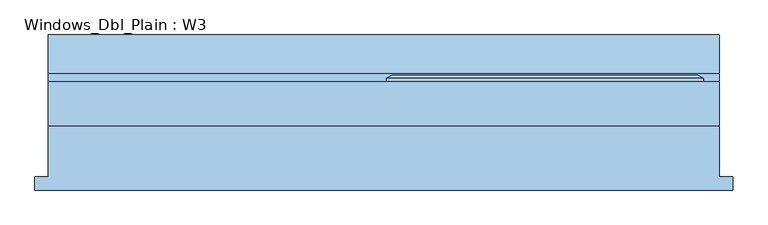
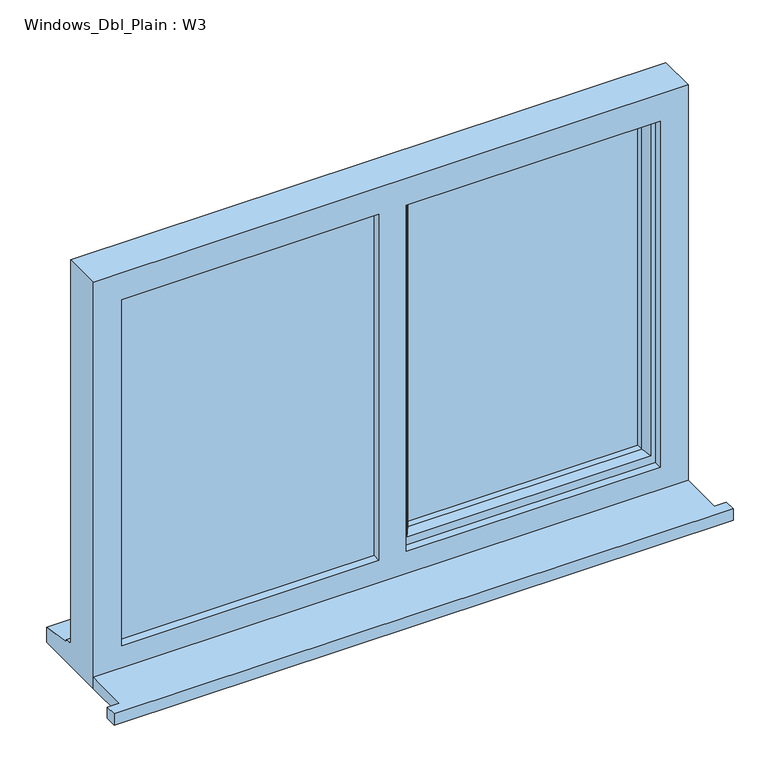
"""IFC4 building model written with IfcOpenShell, lengths in millimetres: window geometry, Windows_Dbl_Plain : W3."""

from ifc_helpers import new_model, si_unit, frame, origin, place, context, project, spatial, polyline, outline, extrude, faceted_brep, source, transform, mapped, element, save


def windows_dbl_plain_w3_a138f75b(model_context):
    return source(origin(), model_context, "Body", "SolidModel", [
        extrude(outline(polyline([(-940.3264, -130.8434322), (-940.3264, -105.8434322), (-915.3264, -105.8434322), (-915.3264, -10.2434322), (345.3264, -10.2434322), (345.3264, -105.8434322), (370.3264, -105.8434322), (370.3264, -130.8434322), (-940.3264, -130.8434322)])), frame((0.0, 0.0, 1200.0), z_axis=(0.0, 0.0, 1.0), x_axis=(1.0, 0.0, 0.0)), (0.0, 0.0, 1.0), 25.0),
        faceted_brep([(-280.0, 72.7565678, 2080.0), (-280.0, 78.5300705, 2080.0), (-280.0, 78.5300705, 1253.0), (-280.0, 72.7565678, 1253.0), (-270.0, 7.7565678, 2070.0), (-270.0, 72.7565678, 2070.0), (-270.0, 72.7565678, 1263.0), (-270.0, 7.7565678, 1263.0), (-230.0, 22.2494677, 2030.0), (-240.1480377, 7.7565678, 2040.1480377), (-240.1480377, 7.7565678, 1292.8519623), (-230.0, 22.2494677, 1303.0), (-230.0, 36.7565678, 2030.0), (-230.0, 36.7565678, 1303.0), (-240.0, 60.7565678, 2040.0), (-240.0, 36.7565678, 2040.0), (-240.0, 36.7565678, 1293.0), (-240.0, 60.7565678, 1293.0), (-230.0, 78.5300705, 2030.0), (-230.0, 60.7565678, 2030.0), (-230.0, 60.7565678, 1303.0), (-230.0, 78.5300705, 1303.0), (-247.4457548, 84.3035732, 2047.4457548), (-247.4457548, 84.3035732, 1285.5542452), (-269.2153903, 84.3035732, 2069.2153903), (-269.2153903, 84.3035732, 1263.7846097), (315.3264, 78.5300705, 1253.0), (315.3264, 72.7565678, 1253.0), (305.3264, 72.7565678, 1263.0), (305.3264, 7.7565678, 1263.0), (275.4744377, 7.7565678, 1292.8519623), (265.3264, 22.2494677, 1303.0), (265.3264, 36.7565678, 1303.0), (275.3264, 36.7565678, 1293.0), (275.3264, 60.7565678, 1293.0), (265.3264, 60.7565678, 1303.0), (265.3264, 78.5300705, 1303.0), (282.7721548, 84.3035732, 1285.5542452), (304.5417903, 84.3035732, 1263.7846097), (315.3264, 78.5300705, 2080.0), (315.3264, 72.7565678, 2080.0), (305.3264, 72.7565678, 2070.0), (305.3264, 7.7565678, 2070.0), (275.4744377, 7.7565678, 2040.1480377), (265.3264, 22.2494677, 2030.0), (265.3264, 36.7565678, 2030.0), (275.3264, 36.7565678, 2040.0), (275.3264, 60.7565678, 2040.0), (265.3264, 60.7565678, 2030.0), (265.3264, 78.5300705, 2030.0), (282.7721548, 84.3035732, 2047.4457548), (304.5417903, 84.3035732, 2069.2153903)], [[[0, 1, 2, 3]], [[4, 5, 6, 7]], [[8, 9, 10, 11]], [[12, 8, 11, 13]], [[14, 15, 16, 17]], [[18, 19, 20, 21]], [[22, 18, 21, 23]], [[1, 24, 25, 2]], [[3, 2, 26, 27]], [[7, 6, 28, 29]], [[11, 10, 30, 31]], [[13, 11, 31, 32]], [[17, 16, 33, 34]], [[21, 20, 35, 36]], [[23, 21, 36, 37]], [[2, 25, 38, 26]], [[27, 26, 39, 40]], [[29, 28, 41, 42]], [[31, 30, 43, 44]], [[32, 31, 44, 45]], [[34, 33, 46, 47]], [[36, 35, 48, 49]], [[37, 36, 49, 50]], [[26, 38, 51, 39]], [[40, 39, 1, 0]], [[3, 27, 40, 0], [5, 41, 28, 6]], [[42, 41, 5, 4]], [[7, 29, 42, 4], [9, 43, 30, 10]], [[44, 43, 9, 8]], [[45, 44, 8, 12]], [[15, 46, 33, 16], [13, 32, 45, 12]], [[47, 46, 15, 14]], [[17, 34, 47, 14], [19, 48, 35, 20]], [[49, 48, 19, 18]], [[50, 49, 18, 22]], [[24, 51, 38, 25], [23, 37, 50, 22]], [[39, 51, 24, 1]]]),
        extrude(outline(polyline([(2050.0, -310.0), (2070.0, -310.0), (2070.0, -875.3264), (1263.0, -875.3264), (1263.0, -310.0), (1283.0, -310.0), (1283.0, -855.3264), (2050.0, -855.3264), (2050.0, -310.0)])), frame((0.0, 31.7565678, 0.0), z_axis=(0.0, 1.0, 0.0), x_axis=(0.0, 0.0, 1.0)), (0.0, 0.0, 1.0), 41.0),
        faceted_brep([(345.3264, -10.2434322, 2110.0), (-915.3264, -10.2434322, 2110.0), (-915.3264, -10.2434322, 1200.0), (345.3264, -10.2434322, 1200.0), (285.3264, -10.2434322, 2050.0), (285.3264, -10.2434322, 1275.0), (-252.0, -10.2434322, 1275.0), (-252.0, -10.2434322, 2050.0), (-310.0, -10.2434322, 2050.0), (-310.0, -10.2434322, 1275.0), (-855.3264, -10.2434322, 1275.0), (-855.3264, -10.2434322, 2050.0), (-915.3264, 72.7565678, 2110.0), (-915.3264, 72.7565678, 1251.0), (-915.3264, 87.7565678, 1249.68767), (-915.3264, 87.7565678, 1244.7449676), (-915.3264, 160.2565678, 1233.8088847), (-915.3264, 160.2565678, 1200.0), (345.3264, 72.7565678, 2110.0), (345.3264, 72.7565678, 1251.0), (-875.3264, 72.7565678, 2070.0), (-875.3264, 72.7565678, 1263.0), (-310.0, 72.7565678, 1263.0), (-310.0, 72.7565678, 2070.0), (-270.0, 72.7565678, 2070.0), (-270.0, 72.7565678, 1263.0), (305.3264, 72.7565678, 1263.0), (305.3264, 72.7565678, 2070.0), (-875.3264, 7.7565678, 2070.0), (-875.3264, 7.7565678, 1263.0), (-300.0, 7.7565678, 2070.0), (-300.0, 7.7565678, 1263.0), (-310.0, 7.7565678, 2050.0), (-855.3264, 7.7565678, 2050.0), (-855.3264, 7.7565678, 1275.0), (-310.0, 7.7565678, 1275.0), (-270.0, 7.7565678, 2070.0), (305.3264, 7.7565678, 2070.0), (305.3264, 7.7565678, 1263.0), (-270.0, 7.7565678, 1263.0), (285.3264, 7.7565678, 2050.0), (-252.0, 7.7565678, 2050.0), (-252.0, 7.7565678, 1275.0), (285.3264, 7.7565678, 1275.0), (-310.0, 31.7565678, 2070.0), (-300.0, 31.7565678, 2070.0), (345.3264, 160.2565678, 1200.0), (345.3264, 160.2565678, 1233.8088847), (345.3264, 87.7565678, 1244.7449676), (345.3264, 87.7565678, 1249.68767), (-300.0, 31.7565678, 1263.0), (-310.0, 31.7565678, 1263.0)], [[[0, 1, 2, 3], [4, 5, 6, 7], [8, 9, 10, 11]], [[2, 1, 12, 13, 14, 15, 16, 17]], [[13, 12, 18, 19], [20, 21, 22, 23], [24, 25, 26, 27]], [[21, 20, 28, 29]], [[28, 30, 31, 29], [32, 33, 34, 35]], [[36, 37, 38, 39], [40, 41, 42, 43]], [[33, 11, 10, 34]], [[1, 0, 18, 12]], [[28, 20, 23, 44, 45, 30]], [[27, 37, 36, 24]], [[11, 33, 32, 8]], [[40, 4, 7, 41]], [[19, 18, 0, 3, 46, 47, 48, 49]], [[27, 26, 38, 37]], [[4, 40, 43, 5]], [[45, 50, 31, 30]], [[50, 45, 44, 51]], [[51, 44, 23, 22]], [[25, 24, 36, 39]], [[41, 7, 6, 42]], [[8, 32, 35, 9]], [[46, 3, 2, 17]], [[47, 46, 17, 16]], [[48, 47, 16, 15]], [[49, 48, 15, 14]], [[19, 49, 14, 13]], [[22, 21, 29, 31, 50, 51]], [[26, 25, 39, 38]], [[6, 5, 43, 42]], [[35, 34, 10, 9]]]),
        extrude(outline(polyline([(-875.3264, 31.7565678), (-300.0, 31.7565678), (-300.0, 7.7565678), (-875.3264, 7.7565678), (-875.3264, 31.7565678)])), frame((0.0, 0.0, 1263.0), z_axis=(0.0, 0.0, 1.0), x_axis=(1.0, 0.0, 0.0)), (0.0, 0.0, 1.0), 807.0),
        extrude(outline(polyline([(275.3264, 36.7565678), (-240.0, 36.7565678), (-240.0, 60.7565678), (275.3264, 60.7565678), (275.3264, 36.7565678)])), frame((0.0, 0.0, 1293.0), z_axis=(0.0, 0.0, 1.0), x_axis=(1.0, 0.0, 0.0)), (0.0, 0.0, 1.0), 747.0),
    ])


if __name__ == "__main__":
    model = new_model("IFC4")
    model_context = context("Model", 3, world=origin())
    ifc_project = project(units=[si_unit("LENGTHUNIT", "METRE", prefix="MILLI")], contexts=[model_context])
    site = spatial("IfcSite", under=ifc_project)
    building = spatial("IfcBuilding", under=site)
    placement = place(None, origin())
    windows_dbl_plain_w3_shape = windows_dbl_plain_w3_a138f75b(model_context)
    element("IfcWindow", 1, ObjectType="Windows_Dbl_Plain : W3", at=placement, inside=building, context=model_context, shape_type="MappedRepresentation", body=[
        mapped(windows_dbl_plain_w3_shape, transform((0.0, 0.0, 0.0), x_axis=(1.0, 0.0, 0.0), y_axis=(0.0, 1.0, 0.0), z_axis=(0.0, 0.0, 1.0))),
    ])
    save(model, "model.ifc")

# Revit data of these elements
# Type "Windows_Dbl_Plain : W3"
#   Type Mark = "59"
#   Operation = "DoublePanelVertical"
#   Construction Type Id = "GSP4R"
#   Manufacturer = "Revit"
#   Keynote = "L10"
#   Analytic Construction = "1/8 in Pilkington single glazing"
#   Wrap Layers (Ext) from Ext = 0.336286 ft
#   Wrap Layers (Int) from Ext = 0.582349 ft
#   Window Board Projection = 0.082021 ft
#   Window Board Extension = 0.082021 ft
#   Visual Light Transmittance = 0.9
#   Solar Heat Gain Coefficient = 0.78
#   Rough Width = 4.136 ft
#   Rough Height = 2.985564 ft
#   Height = 2.985564 ft
#   Width = 4.136 ft
#   Heat Transfer Coefficient (U) = 3.6886 W/(m²·K)
#   Glazing Thickness = 0.07874 ft
#   FrameOffset - External = 0.164042 ft
#   Frame Depth = 0.213255 ft
#   Default Head Height = 6.922572 ft
#   Cill Depth = 0.287073 ft
#   Cavity Closer Width = 0.164042 ft
#   Cavity Closer Offset from Ext = 0.336286 ft
#   Cavity Closer Depth = 0.278871 ft
#   Vis - Cavity Closers = yes
#   Define Thermal Properties by = 1
#   Material Trim = Window Frame
#   Material Glass = Glass
#   Material Frame = Cherry
#   Wall Closure = (empty or 0)
# Element 1 (IfcWindow, "Windows_Dbl_Plain : W3")
#   Materials on its faces: "Cherry", "Glass", "Window Frame"
# Materials
#   "Window Frame": colour RGB 249 249 249, transparency 0, Keynote = "L10", Cost = 0
#   "Glass": class "Glass", colour RGB 0 128 192, transparency 0.9, Description = "Soda Lime Glass", Cost = 0
#   "Cherry": class "Wood", colour RGB 226 177 128, transparency 0, Description = "Prunus Serotina", Cost = 0
